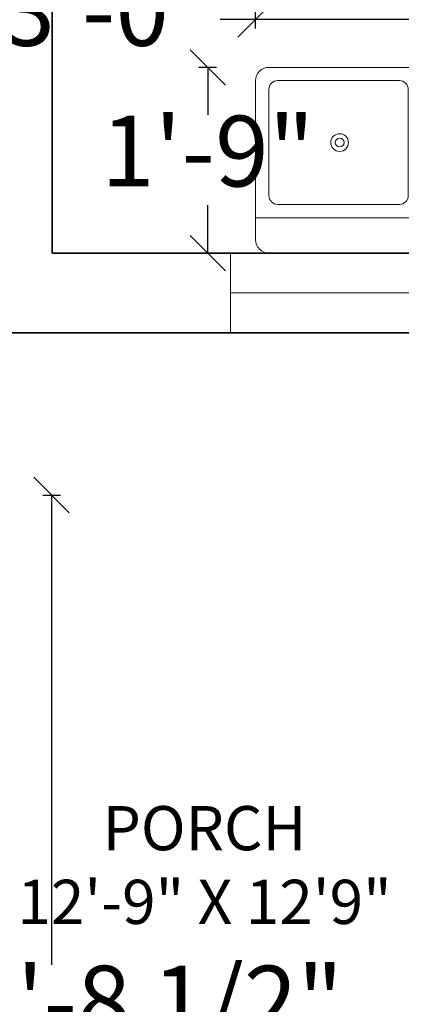
# Model space of a CAD drawing. Units: inches. Extents: x 2558 to 3026, y 433 to 1053.
# Tile 5 of 8: x 2877 to 2921, y 574 to 685. Entities that reach past the tile are written whole.
import ezdxf

# ---------------------------------------------------------------- set-up
doc = ezdxf.new("R2010")
doc.units = ezdxf.units.IN
for name, color, linetype, lineweight in [('A-ANNO-DIMS', 2, 'Continuous', 18), ('A-AREA-IDEN', 7, 'Continuous', 18), ('A-FLOR-FIXT', 9, 'Continuous', 18), ('A-GLAZ', 5, 'Continuous', 18), ('A-WALL', 7, 'Continuous', 35)]:
    doc.layers.add(name, color=color, linetype=linetype, lineweight=lineweight)
doc.styles.get("Standard").update_dxf_attribs({"font": 'arial.ttf'})
doc.dimstyles.new('ISO-25', dxfattribs={"dimtxt": 8, "dimasz": 4, "dimexe": 1, "dimexo": 1, "dimgap": 1, "dimtad": 0, "dimtih": 1, "dimtoh": 1, "dimlunit": 3, "dimtxsty": 'Standard', "dimblk": 'OBLIQUE', "dimcen": 2.5, "dimclrt": 1, "dimadec": 0, "dimazin": 0, "dimtfac": 1, "dimtmove": 0, "dimatfit": 3, "dimfxl": 1, "dimfxlon": 1, "dimarcsym": 0})

# ---------------------------------------------------------------- blocks, each defined once
blk = doc.blocks.new('Sink-double - 36 in top')
for p, q in [((-18, -4), (18, -4)), ((-0.75, -18.5), (-0.75, -6.5)), ((0.75, -6.5), (0.75, -18.5))]:
    blk.add_line(p, q)
for points in [[(-16.5, 0), (16.5, 0)], [(-18, -19.5), (-18, -1.5)], [(18, -1.5), (18, -19.5)], [(-15.5, -5.5), (-1.75, -5.5)], [(1.75, -5.5), (15.5, -5.5)], [(-16.5, -18.5), (-16.5, -6.5)], [(16.5, -6.5), (16.5, -18.5)], [(-1.75, -19.5), (-15.5, -19.5)], [(15.5, -19.5), (1.75, -19.5)], [(16.5, -21), (-16.5, -21)]]:
    blk.add_lwpolyline(points)
for centre, radius in [((-8.5, -12.5), 1), ((-8.5, -12.5), 0.5), ((8.5, -12.5), 1), ((8.5, -12.5), 0.5)]:
    blk.add_circle(centre, radius)
for centre, radius, start, end in [((-16.5, -1.5), 1.5, 90, 180), ((16.5, -1.5), 1.5, 0, 90), ((-15.5, -6.5), 1, 90, 180), ((-1.75, -6.5), 1, 0, 90), ((1.75, -6.5), 1, 90, 180), ((15.5, -6.5), 1, 0, 90), ((-15.5, -18.5), 1, 180, 270), ((-1.75, -18.5), 1, 270, 0), ((1.75, -18.5), 1, 180, 270), ((15.5, -18.5), 1, 270, 0), ((-16.5, -19.5), 1.5, 180, 270), ((16.5, -19.5), 1.5, 270, 0)]:
    blk.add_arc(centre, radius, start, end)
blk = doc.blocks.new('_Oblique')
at = {"color": 0, "linetype": 'ByBlock', "lineweight": -2}
blk.add_line((-0.5, -0.5), (0.5, 0.5), dxfattribs=at)
blk = doc.blocks.new('*D41')
at = {"layer": 'A-ANNO-DIMS', "color": 0, "lineweight": -2, "transparency": 16777216}
for p, q in [((2904.13, 684.22), (2904.13, 686.22)), ((2940.13, 684.22), (2940.13, 686.22)), ((2904.13, 685.22), (2900.13, 685.22)), ((2940.13, 685.22), (2904.13, 685.22))]:
    blk.add_line(p, q, dxfattribs=at)
at = {"layer": 'Defpoints', "color": 0, "transparency": 16777216}
for p in [(2904.13, 685.22), (2904.13, 679.82), (2940.13, 679.82)]:
    blk.add_point(p, dxfattribs=at)
at = {"layer": 'A-ANNO-DIMS', "color": 0, "lineweight": -2, "transparency": 16777216, "xscale": 4, "yscale": 4, "zscale": 4, "rotation": 180}
blk.add_blockref('_Oblique', (2904.13, 685.22), dxfattribs=at)
at = {"layer": 'A-ANNO-DIMS', "color": 0, "lineweight": -2, "transparency": 16777216, "xscale": 4, "yscale": 4, "zscale": 4}
blk.add_blockref('_Oblique', (2940.13, 685.22), dxfattribs=at)
at = {"layer": 'A-ANNO-DIMS', "color": 1, "transparency": 16777216, "insert": (2873.92, 685.22), "char_height": 8, "attachment_point": 5}
blk.add_mtext('SINK 3\'-0"', dxfattribs=at)
blk = doc.blocks.new('*D42')
at = {"layer": 'A-ANNO-DIMS', "color": 0, "lineweight": -2, "transparency": 16777216}
for p, q in [((2899.73, 679.82), (2897.73, 679.82)), ((2898.73, 679.82), (2898.73, 674.41)), ((2898.73, 658.82), (2898.73, 664.24)), ((2899.73, 658.82), (2897.73, 658.82))]:
    blk.add_line(p, q, dxfattribs=at)
at = {"layer": 'Defpoints', "color": 0, "transparency": 16777216}
for p in [(2904.13, 679.82), (2898.73, 658.82), (2904.13, 658.82)]:
    blk.add_point(p, dxfattribs=at)
at = {"layer": 'A-ANNO-DIMS', "color": 0, "lineweight": -2, "transparency": 16777216, "xscale": 4, "yscale": 4, "zscale": 4}
for p, rotation in [((2898.73, 679.82), 90), ((2898.73, 658.82), 270)]:
    blk.add_blockref('_Oblique', p, dxfattribs=dict(at, rotation=rotation))
at = {"layer": 'A-ANNO-DIMS', "color": 1, "transparency": 16777216, "insert": (2898.73, 669.32), "char_height": 8, "attachment_point": 5}
blk.add_mtext('1\'-9"', dxfattribs=at)
blk = doc.blocks.new('*D43')
at = {"layer": 'A-ANNO-DIMS', "color": 0, "lineweight": -2, "transparency": 16777216}
for p, q in [((2880.07, 631.47), (2882.07, 631.47)), ((2881.07, 631.47), (2881.07, 578.35)), ((2881.07, 514.96), (2881.07, 568.08)), ((2880.07, 514.96), (2882.07, 514.96))]:
    blk.add_line(p, q, dxfattribs=at)
at = {"layer": 'Defpoints', "color": 0, "transparency": 16777216}
for p in [(2863.59, 631.47), (2881.07, 631.47), (2863.59, 514.96)]:
    blk.add_point(p, dxfattribs=at)
at = {"layer": 'A-ANNO-DIMS', "color": 0, "lineweight": -2, "transparency": 16777216, "xscale": 4, "yscale": 4, "zscale": 4}
for p, rotation in [((2881.07, 631.47), 90), ((2881.07, 514.96), 270)]:
    blk.add_blockref('_Oblique', p, dxfattribs=dict(at, rotation=rotation))
at = {"layer": 'A-ANNO-DIMS', "color": 1, "transparency": 16777216, "insert": (2881.07, 573.21), "char_height": 8, "attachment_point": 5}
blk.add_mtext('CAR 9\'-8 1/2"', dxfattribs=at)
blk = doc.blocks.new('*D58')
at = {"layer": 'A-ANNO-DIMS', "color": 0, "lineweight": -2, "transparency": 16777216}
for p, q in [((2901.29, 1039.77), (2901.29, 1041.77)), ((2943.34, 1039.77), (2943.34, 1041.77)), ((2901.29, 1040.77), (2910.69, 1040.77)), ((2943.34, 1040.77), (2933.95, 1040.77))]:
    blk.add_line(p, q, dxfattribs=at)
at = {"layer": 'Defpoints', "color": 0, "transparency": 16777216}
for p in [(2943.34, 1040.77), (2901.29, 649.82), (2943.34, 649.82)]:
    blk.add_point(p, dxfattribs=at)
at = {"layer": 'A-ANNO-DIMS', "color": 0, "lineweight": -2, "transparency": 16777216, "xscale": 4, "yscale": 4, "zscale": 4, "rotation": 180}
blk.add_blockref('_Oblique', (2901.29, 1040.77), dxfattribs=at)
at = {"layer": 'A-ANNO-DIMS', "color": 0, "lineweight": -2, "transparency": 16777216, "xscale": 4, "yscale": 4, "zscale": 4}
blk.add_blockref('_Oblique', (2943.34, 1040.77), dxfattribs=at)
at = {"layer": 'A-ANNO-DIMS', "color": 1, "transparency": 16777216, "insert": (2922.32, 1040.77), "char_height": 8, "attachment_point": 5}
blk.add_mtext('3\'-6"', dxfattribs=at)
blk = doc.blocks.new('*D60')
at = {"layer": 'A-ANNO-DIMS', "color": 0, "lineweight": -2, "transparency": 16777216}
for p, q in [((2996.58, 575.69), (2998.58, 575.69)), ((2997.58, 575.69), (2997.58, 562.78)), ((2997.58, 539.69), (2997.58, 552.6)), ((2996.58, 539.69), (2998.58, 539.69))]:
    blk.add_line(p, q, dxfattribs=at)
at = {"layer": 'Defpoints', "color": 0, "transparency": 16777216}
for p in [(2807.63, 575.69), (2997.58, 575.69), (2807.63, 539.69)]:
    blk.add_point(p, dxfattribs=at)
at = {"layer": 'A-ANNO-DIMS', "color": 0, "lineweight": -2, "transparency": 16777216, "xscale": 4, "yscale": 4, "zscale": 4}
for p, rotation in [((2997.58, 575.69), 90), ((2997.58, 539.69), 270)]:
    blk.add_blockref('_Oblique', p, dxfattribs=dict(at, rotation=rotation))
at = {"layer": 'A-ANNO-DIMS', "color": 1, "transparency": 16777216, "insert": (2997.58, 557.69), "char_height": 8, "attachment_point": 5}
blk.add_mtext('3\'-0"', dxfattribs=at)
blk = doc.blocks.new('*D73')
at = {"layer": 'A-ANNO-DIMS', "color": 0, "lineweight": -2, "transparency": 16777216}
for p, q in [((2816.63, 1039.77), (2816.63, 1041.77)), ((2959.63, 1039.77), (2959.63, 1041.77)), ((2816.63, 1040.77), (2870.66, 1040.77)), ((2959.63, 1040.77), (2905.6, 1040.77))]:
    blk.add_line(p, q, dxfattribs=at)
at = {"layer": 'Defpoints', "color": 0, "transparency": 16777216}
for p in [(2959.63, 1040.77), (2816.63, 481.83), (2959.63, 481.82)]:
    blk.add_point(p, dxfattribs=at)
at = {"layer": 'A-ANNO-DIMS', "color": 0, "lineweight": -2, "transparency": 16777216, "xscale": 4, "yscale": 4, "zscale": 4, "rotation": 180}
blk.add_blockref('_Oblique', (2816.63, 1040.77), dxfattribs=at)
at = {"layer": 'A-ANNO-DIMS', "color": 0, "lineweight": -2, "transparency": 16777216, "xscale": 4, "yscale": 4, "zscale": 4}
blk.add_blockref('_Oblique', (2959.63, 1040.77), dxfattribs=at)
at = {"layer": 'A-ANNO-DIMS', "color": 1, "transparency": 16777216, "insert": (2888.13, 1040.77), "char_height": 8, "attachment_point": 5}
blk.add_mtext('11\'-11"', dxfattribs=at)
blk = doc.blocks.new('*D75')
at = {"layer": 'A-ANNO-DIMS', "color": 0, "lineweight": -2, "transparency": 16777216}
for p, q in [((2831.63, 445.87), (2831.63, 443.87)), ((2839.13, 445.87), (2839.13, 443.87)), ((2831.63, 444.87), (2839.13, 444.87)), ((2839.13, 444.87), (2843.13, 444.87))]:
    blk.add_line(p, q, dxfattribs=at)
at = {"layer": 'Defpoints', "color": 0, "transparency": 16777216}
for p in [(2831.63, 799.82), (2839.13, 799.82), (2839.13, 444.87)]:
    blk.add_point(p, dxfattribs=at)
at = {"layer": 'A-ANNO-DIMS', "color": 0, "lineweight": -2, "transparency": 16777216, "xscale": 4, "yscale": 4, "zscale": 4, "rotation": 180}
blk.add_blockref('_Oblique', (2831.63, 444.87), dxfattribs=at)
at = {"layer": 'A-ANNO-DIMS', "color": 0, "lineweight": -2, "transparency": 16777216, "xscale": 4, "yscale": 4, "zscale": 4}
blk.add_blockref('_Oblique', (2839.13, 444.87), dxfattribs=at)
at = {"layer": 'A-ANNO-DIMS', "color": 1, "transparency": 16777216, "insert": (2864.09, 444.87), "char_height": 8, "attachment_point": 5}
blk.add_mtext('0\'-7 1/2"', dxfattribs=at)
blk = doc.blocks.new('*D76')
at = {"layer": 'A-ANNO-DIMS', "color": 0, "lineweight": -2, "transparency": 16777216}
for p, q in [((2879.03, 445.87), (2879.03, 443.87)), ((2911.03, 445.87), (2911.03, 443.87)), ((2879.03, 444.87), (2883.32, 444.87)), ((2911.03, 444.87), (2906.73, 444.87))]:
    blk.add_line(p, q, dxfattribs=at)
at = {"layer": 'Defpoints', "color": 0, "transparency": 16777216}
for p in [(2879.03, 943.82), (2911.03, 943.82), (2911.03, 444.87)]:
    blk.add_point(p, dxfattribs=at)
at = {"layer": 'A-ANNO-DIMS', "color": 0, "lineweight": -2, "transparency": 16777216, "xscale": 4, "yscale": 4, "zscale": 4, "rotation": 180}
blk.add_blockref('_Oblique', (2879.03, 444.87), dxfattribs=at)
at = {"layer": 'A-ANNO-DIMS', "color": 0, "lineweight": -2, "transparency": 16777216, "xscale": 4, "yscale": 4, "zscale": 4}
blk.add_blockref('_Oblique', (2911.03, 444.87), dxfattribs=at)
at = {"layer": 'A-ANNO-DIMS', "color": 1, "transparency": 16777216, "insert": (2895.03, 444.87), "char_height": 8, "attachment_point": 5}
blk.add_mtext('2\'-8"', dxfattribs=at)
blk = doc.blocks.new('*D77')
at = {"layer": 'A-ANNO-DIMS', "color": 0, "lineweight": -2, "transparency": 16777216}
for p, q in [((2867.63, 445.87), (2867.63, 443.87)), ((2875.13, 445.87), (2875.13, 443.87)), ((2867.63, 444.87), (2875.13, 444.87)), ((2875.13, 444.87), (2879.13, 444.87))]:
    blk.add_line(p, q, dxfattribs=at)
at = {"layer": 'Defpoints', "color": 0, "transparency": 16777216}
for p in [(2867.63, 658.82), (2875.13, 658.82), (2875.13, 444.87)]:
    blk.add_point(p, dxfattribs=at)
at = {"layer": 'A-ANNO-DIMS', "color": 0, "lineweight": -2, "transparency": 16777216, "xscale": 4, "yscale": 4, "zscale": 4, "rotation": 180}
blk.add_blockref('_Oblique', (2867.63, 444.87), dxfattribs=at)
at = {"layer": 'A-ANNO-DIMS', "color": 0, "lineweight": -2, "transparency": 16777216, "xscale": 4, "yscale": 4, "zscale": 4}
blk.add_blockref('_Oblique', (2875.13, 444.87), dxfattribs=at)
at = {"layer": 'A-ANNO-DIMS', "color": 1, "transparency": 16777216, "insert": (2900.09, 444.87), "char_height": 8, "attachment_point": 5}
blk.add_mtext('0\'-7 1/2"', dxfattribs=at)

msp = doc.modelspace()

# ---------------------------------------------------------------- linework, layer by layer
at = {"layer": 'A-GLAZ'}
for p, q in [((2901.294, 658.825), (2901.294, 649.825)), ((2901.294, 654.325), (2943.344, 654.325))]:
    msp.add_line(p, q, dxfattribs=at)
at = {"layer": 'A-WALL'}
for p, q in [((2881.133, 658.825), (2881.133, 753.433)), ((2960.633, 658.825), (2881.133, 658.825)), ((2960.633, 649.825), (2867.633, 649.825))]:
    msp.add_line(p, q, dxfattribs=at)

# ---------------------------------------------------------------- block references
at = {"layer": 'A-FLOR-FIXT', "rotation": 180}
msp.add_blockref('Sink-double - 36 in top', (2922.13, 658.825), dxfattribs=at)

# ---------------------------------------------------------------- texts
at = {"layer": 'A-AREA-IDEN', "insert": (2872.093, 596.302), "char_height": 5, "attachment_point": 1}
msp.add_mtext_dynamic_manual_height_columns('\\pxqc;PORCH\\P12\'-9" X 12\'9"', width=52.53987, gutter_width=12.5, heights=[0], dxfattribs=at)

# ---------------------------------------------------------------- dimensions: what is measured, and where the dimension line sits
at = {"layer": 'A-ANNO-DIMS'}
for base, p1, p2, picture, middle in [((2959.633, 1040.775), (2816.633, 481.827), (2959.633, 481.825), '*D73', (2888.133, 1040.775)), ((2943.3439, 1040.7746), (2901.2944, 649.8246), (2943.3439, 649.8246), '*D58', (2922.3191, 1040.7746)), ((2911.025, 444.875), (2879.025, 943.825), (2911.025, 943.825), '*D76', (2895.025, 444.875)), ((2839.133, 444.875), (2831.633, 799.825), (2839.133, 799.825), '*D75', (2864.086, 444.875)), ((2875.133, 444.875), (2867.633, 658.825), (2875.133, 658.825), '*D77', (2900.086, 444.875))]:
    dim = msp.add_linear_dim(base=base, p1=p1, p2=p2, dimstyle='ISO-25', override={"dimdec": 1, "dimlfac": 1, "dimrnd": 0, "dimzin": 1, "dimdsep": 46, "dimlunit": 4, "dimfrac": 2}, dxfattribs=at)
    dim.commit()
    dim.dimension.update_dxf_attribs({"geometry": picture, "text_midpoint": middle})
for base, p1, p2, angle, text, picture, middle in [((2904.13, 685.225), (2940.13, 679.825), (2904.13, 679.825), 180, 'SINK <>', '*D41', (2873.922, 685.225)), ((2881.069, 631.468), (2863.592, 514.956), (2863.592, 631.468), 90, 'CAR <>', '*D43', (2881.069, 573.212))]:
    dim = msp.add_linear_dim(base=base, p1=p1, p2=p2, angle=angle, text=text, dimstyle='ISO-25', override={"dimdec": 1, "dimlfac": 1, "dimrnd": 0, "dimzin": 1, "dimdsep": 46, "dimlunit": 4, "dimfrac": 2}, dxfattribs=at)
    dim.commit()
    dim.dimension.update_dxf_attribs({"geometry": picture, "text_midpoint": middle})
for base, p1, p2, angle, picture, middle in [((2898.73, 658.825), (2904.13, 679.825), (2904.13, 658.825), 270, '*D42', (2898.73, 669.325)), ((2997.583, 575.691), (2807.633, 539.691), (2807.633, 575.691), 90, '*D60', (2997.583, 557.691))]:
    dim = msp.add_linear_dim(base=base, p1=p1, p2=p2, angle=angle, dimstyle='ISO-25', override={"dimdec": 1, "dimlfac": 1, "dimrnd": 0, "dimzin": 1, "dimdsep": 46, "dimlunit": 4, "dimfrac": 2}, dxfattribs=at)
    dim.commit()
    dim.dimension.update_dxf_attribs({"geometry": picture, "text_midpoint": middle})

doc.saveas('drawing.dxf')
